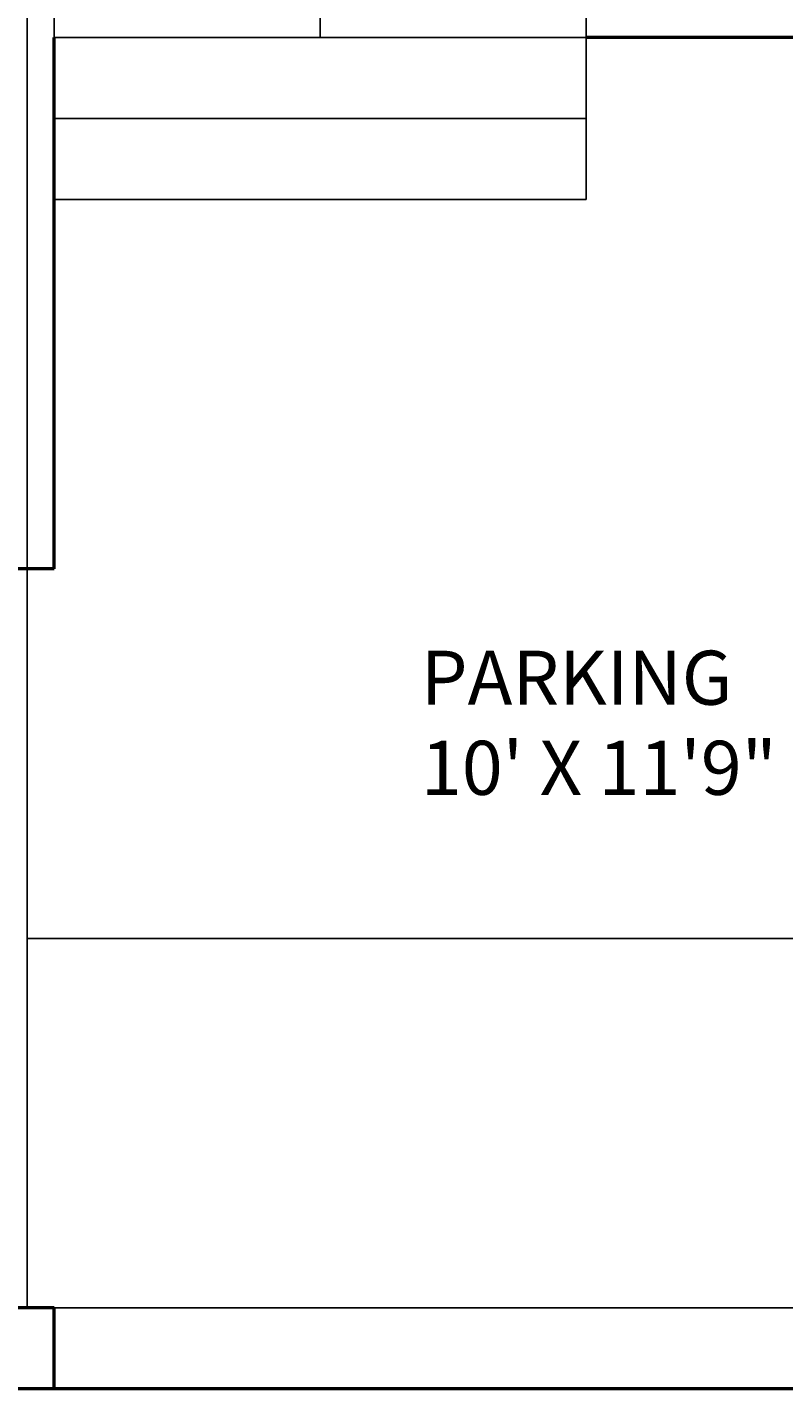
# Model space of a CAD drawing. Units: inches. Extents: x 37 to 824, y -700 to 234.
# Tile 37 of 77: x 296 to 380, y -366 to -215. Entities that reach past the tile are written whole.
import ezdxf

# ---------------------------------------------------------------- set-up
doc = ezdxf.new("R2010")
doc.units = ezdxf.units.IN
doc.header["$MEASUREMENT"] = 0
for name, color, linetype, lineweight in [('A-ANNO-DIMS', 2, 'Continuous', 18), ('A-AREA-IDEN', 3, 'Continuous', 18), ('A-DOOR', 4, 'Continuous', 25), ('A-FLOR-STRS', 1, 'Continuous', 25), ('A-WALL', 2, 'Continuous', 50)]:
    doc.layers.add(name, color=color, linetype=linetype, lineweight=lineweight)
doc.styles.get("Standard").update_dxf_attribs({"font": 'arial.ttf'})
doc.dimstyles.get("Standard").update_dxf_attribs({"dimtxt": 0.18, "dimasz": 0.18, "dimexe": 0.18, "dimexo": 0.0625, "dimgap": 0.09, "dimtad": 0, "dimtih": 1, "dimtoh": 1, "dimdec": 1, "dimzin": 0, "dimdsep": 46, "dimlunit": 4, "dimtxsty": 'Standard', "dimcen": 0.09, "dimadec": 0, "dimazin": 0, "dimtfac": 1, "dimtdec": 1, "dimtofl": 0, "dimtmove": 0, "dimatfit": 3, "dimfxl": 1, "dimtolj": 1, "dimtzin": 0, "dimarcsym": 0})

# ---------------------------------------------------------------- blocks, each defined once
blk = doc.blocks.new('*U4')
for p, q in [((0, 0), (0, -100)), ((750, 0), (750, -100))]:
    blk.add_line(p, q)
blk.add_lwpolyline([(0, 0), (0, 750), (43.75, 750), (43.75, 0)], close=True)
blk.add_arc((0, 0), 750, 0, 90)
blk = doc.blocks.new('*D87')
at = {"layer": 'A-ANNO-DIMS', "color": 0, "lineweight": -2, "ltscale": 0.5, "transparency": 16777216}
for p, q in [((216.08, -356.85), (216.08, 234.17)), ((216.26, 233.99), (255.75, 233.99)), ((295.9, 233.99), (256.41, 233.99)), ((296.08, -356.85), (296.08, 234.17))]:
    blk.add_line(p, q, dxfattribs=at)
at = {"layer": 'A-ANNO-DIMS', "color": 0, "ltscale": 0.5, "transparency": 16777216}
for points in [[(216.26, 234.02), (216.26, 233.96), (216.08, 233.99)], [(295.9, 234.02), (295.9, 233.96), (296.08, 233.99)]]:
    blk.add_solid(points, dxfattribs=at)
at = {"layer": 'Defpoints', "color": 0, "ltscale": 0.5, "transparency": 16777216}
for p in [(296.08, 233.99), (216.08, -356.91), (296.08, -356.91)]:
    blk.add_point(p, dxfattribs=at)
at = {"layer": 'A-ANNO-DIMS', "color": 0, "ltscale": 0.5, "transparency": 16777216, "insert": (256.08, 233.99), "char_height": 0.18, "attachment_point": 5}
blk.add_mtext('\\A1;6\'-8"', dxfattribs=at)
blk = doc.blocks.new('*D88')
at = {"layer": 'A-ANNO-DIMS', "color": 0, "lineweight": -2, "ltscale": 0.5, "transparency": 16777216}
for p, q in [((296.14, -315.91), (513.77, -315.91)), ((513.59, -316.09), (513.59, -336.23)), ((513.59, -356.73), (513.59, -336.59)), ((296.14, -356.91), (513.77, -356.91))]:
    blk.add_line(p, q, dxfattribs=at)
at = {"layer": 'A-ANNO-DIMS', "color": 0, "ltscale": 0.5, "transparency": 16777216}
for points in [[(513.56, -316.09), (513.62, -316.09), (513.59, -315.91)], [(513.56, -356.73), (513.62, -356.73), (513.59, -356.91)]]:
    blk.add_solid(points, dxfattribs=at)
at = {"layer": 'Defpoints', "color": 0, "ltscale": 0.5, "transparency": 16777216}
for p in [(296.08, -315.91), (296.08, -356.91), (513.59, -356.91)]:
    blk.add_point(p, dxfattribs=at)
at = {"layer": 'A-ANNO-DIMS', "color": 0, "ltscale": 0.5, "transparency": 16777216, "insert": (513.59, -336.41), "char_height": 0.18, "attachment_point": 5}
blk.add_mtext('\\A1;3\'-5"', dxfattribs=at)

msp = doc.modelspace()

# ---------------------------------------------------------------- linework, layer by layer
at = {"layer": 'A-FLOR-STRS', "ltscale": 0.5}
for p, q in [((358.13, -215.91), (299.08, -215.91)), ((299.08, -215.91), (299.08, -233.91)), ((358.13, -215.91), (358.13, -233.91)), ((358.13, -224.91), (299.08, -224.91)), ((358.13, -233.91), (299.08, -233.91))]:
    msp.add_line(p, q, dxfattribs=at)
at = {"layer": 'A-FLOR-STRS'}
msp.add_line((328.87, -215.91), (328.34, -215.91), dxfattribs=at)
at = {"layer": 'A-WALL'}
for p, q in [((299.08, -274.91), (299.08, -215.91)), ((419.08, -215.91), (358.13, -215.91)), ((299.08, -274.91), (170.08, -274.91)), ((299.08, -356.91), (170.08, -356.91)), ((299.08, -365.91), (299.08, -356.91)), ((428.08, -365.91), (161.08, -365.91))]:
    msp.add_line(p, q, dxfattribs=at)

# ---------------------------------------------------------------- block references
at = {"layer": 'A-DOOR', "yscale": 0.0393700787401575, "zscale": 0.0393700787401575}
for p, xscale in [((299.08, -211.97), 0.0393700787401575), ((358.13, -211.97), -0.0393700787401575)]:
    msp.add_blockref('*U4', p, dxfattribs=dict(at, xscale=xscale))

# ---------------------------------------------------------------- texts
at = {"layer": 'A-AREA-IDEN', "insert": (339.79, -283.98), "char_height": 6, "attachment_point": 1}
msp.add_mtext_dynamic_manual_height_columns('PARKING\\P10\' X 11\'9"', width=88.3217, gutter_width=1, heights=[0], dxfattribs=at)

# ---------------------------------------------------------------- dimensions: what is measured, and where the dimension line sits
at = {"layer": 'A-ANNO-DIMS', "ltscale": 0.5}
dim = msp.add_linear_dim(base=(296.08, 233.99), p1=(216.08, -356.91), p2=(296.08, -356.91), dimstyle='Standard', override={"dimdec": 1, "dimlfac": 1, "dimrnd": 0, "dimzin": 1, "dimdsep": 46, "dimlunit": 4, "dimfrac": 2}, dxfattribs=at)
dim.commit()
dim.dimension.update_dxf_attribs({"geometry": '*D87', "text_midpoint": (256.08, 233.99)})
dim = msp.add_linear_dim(base=(513.59, -356.91), p1=(296.08, -315.91), p2=(296.08, -356.91), angle=90, dimstyle='Standard', override={"dimdec": 1, "dimlfac": 1, "dimrnd": 0, "dimzin": 1, "dimdsep": 46, "dimlunit": 4, "dimfrac": 2}, dxfattribs=at)
dim.commit()
dim.dimension.update_dxf_attribs({"geometry": '*D88', "text_midpoint": (513.59, -336.41)})

doc.saveas('drawing.dxf')
